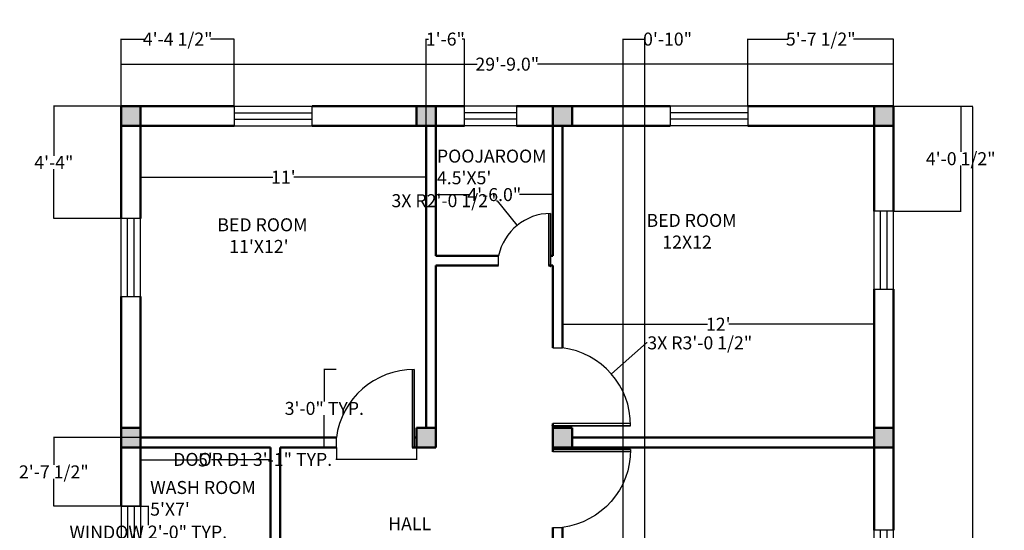
# Model space of a CAD drawing. Units: inches. Extents: x 1935 to 2390, y 6777 to 7449.
# Tile 2 of 2: x 1935 to 2390, y 7213 to 7449. Entities that reach past the tile are written whole.
import ezdxf

# ---------------------------------------------------------------- set-up
doc = ezdxf.new("R2010")
doc.units = ezdxf.units.IN
doc.header["$MEASUREMENT"] = 0
for name, color, linetype, lineweight in [('A-ANNO-DIMS', 7, 'Continuous', 18), ('A-AREA-IDEN', 7, 'Continuous', 25), ('A-COLS', 42, 'Continuous', 50), ('A-COLS-PATT', 7, 'Continuous', 13), ('A-DOOR', 50, 'Continuous', 25), ('A-GLAZ', 140, 'Continuous', 25), ('A-WALL', 42, 'Continuous', 50)]:
    doc.layers.add(name, color=color, linetype=linetype, lineweight=lineweight)
doc.styles.get("Standard").update_dxf_attribs({"font": 'arial.ttf'})
doc.dimstyles.get("Standard").update_dxf_attribs({"dimtxt": 6, "dimasz": 0.18, "dimexe": 0.18, "dimexo": 0.0625, "dimgap": 0.09, "dimtad": 0, "dimtih": 1, "dimtoh": 1, "dimdec": 1, "dimzin": 0, "dimdsep": 46, "dimlunit": 3, "dimtxsty": 'Standard', "dimcen": 0.09, "dimclrd": 200, "dimclre": 200, "dimclrt": 200, "dimadec": 0, "dimazin": 0, "dimtfac": 1, "dimtdec": 1, "dimtofl": 0, "dimtmove": 0, "dimatfit": 3, "dimfxl": 1, "dimtolj": 1, "dimtzin": 0, "dimarcsym": 0})

# ---------------------------------------------------------------- blocks, each defined once
blk = doc.blocks.new('*D1')
at = {"layer": 'A-ANNO-DIMS', "color": 0, "lineweight": -2, "transparency": 16777216}
for p, q in [((1990.87, 7400.15), (1990.87, 7376.35)), ((2122.87, 7400.15), (2122.87, 7376.35)), ((1991.05, 7376.53), (2051.97, 7376.53)), ((2122.69, 7376.53), (2061.76, 7376.53))]:
    blk.add_line(p, q, dxfattribs=at)
at = {"layer": 'A-ANNO-DIMS', "color": 0, "transparency": 16777216}
for points in [[(1991.05, 7376.56), (1991.05, 7376.5), (1990.87, 7376.53)], [(2122.69, 7376.56), (2122.69, 7376.5), (2122.87, 7376.53)]]:
    blk.add_solid(points, dxfattribs=at)
at = {"layer": 'Defpoints', "color": 0, "transparency": 16777216}
for p in [(1990.87, 7400.21), (2122.87, 7400.21), (2122.87, 7376.53)]:
    blk.add_point(p, dxfattribs=at)
at = {"layer": 'A-ANNO-DIMS', "color": 0, "transparency": 16777216, "insert": (2056.87, 7376.53), "char_height": 6, "attachment_point": 5}
blk.add_mtext("\\A1;11'", dxfattribs=at)
blk = doc.blocks.new('*D2')
at = {"layer": 'A-ANNO-DIMS', "color": 0, "lineweight": -2, "transparency": 16777216}
for p, q in [((1990.87, 7251.65), (1990.87, 7245.73)), ((2050.87, 7251.65), (2050.87, 7245.73)), ((1991.05, 7245.91), (2018.02, 7245.91)), ((2050.69, 7245.91), (2023.72, 7245.91))]:
    blk.add_line(p, q, dxfattribs=at)
at = {"layer": 'A-ANNO-DIMS', "color": 0, "transparency": 16777216}
for points in [[(1991.05, 7245.94), (1991.05, 7245.88), (1990.87, 7245.91)], [(2050.69, 7245.94), (2050.69, 7245.88), (2050.87, 7245.91)]]:
    blk.add_solid(points, dxfattribs=at)
at = {"layer": 'Defpoints', "color": 0, "transparency": 16777216}
for p in [(1990.87, 7251.71), (2050.87, 7251.71), (2050.87, 7245.91)]:
    blk.add_point(p, dxfattribs=at)
at = {"layer": 'A-ANNO-DIMS', "color": 0, "transparency": 16777216, "insert": (2020.87, 7245.91), "char_height": 6, "attachment_point": 5}
blk.add_mtext("\\A1;5'", dxfattribs=at)
blk = doc.blocks.new('*D7')
at = {"layer": 'A-ANNO-DIMS', "color": 0, "lineweight": -2, "transparency": 16777216}
for p, q in [((2127.37, 7400.15), (2127.37, 7368.27)), ((2181.37, 7400.15), (2181.37, 7368.27)), ((2127.55, 7368.45), (2142.68, 7368.45)), ((2181.19, 7368.45), (2166.05, 7368.45))]:
    blk.add_line(p, q, dxfattribs=at)
at = {"layer": 'A-ANNO-DIMS', "color": 0, "transparency": 16777216}
for points in [[(2127.55, 7368.48), (2127.55, 7368.42), (2127.37, 7368.45)], [(2181.19, 7368.48), (2181.19, 7368.42), (2181.37, 7368.45)]]:
    blk.add_solid(points, dxfattribs=at)
at = {"layer": 'Defpoints', "color": 0, "transparency": 16777216}
for p in [(2127.37, 7400.21), (2181.37, 7400.21), (2181.37, 7368.45)]:
    blk.add_point(p, dxfattribs=at)
at = {"layer": 'A-ANNO-DIMS', "color": 0, "transparency": 16777216, "insert": (2154.37, 7368.45), "char_height": 6, "attachment_point": 5}
blk.add_mtext('\\A1;4\'-6.0"', dxfattribs=at)
blk = doc.blocks.new('*D8')
at = {"layer": 'A-ANNO-DIMS', "color": 0, "lineweight": -2, "transparency": 16777216}
for p, q in [((2185.87, 7316.65), (2185.87, 7308.4)), ((2329.87, 7316.65), (2329.87, 7308.4)), ((2186.05, 7308.58), (2252.97, 7308.58)), ((2329.69, 7308.58), (2262.76, 7308.58))]:
    blk.add_line(p, q, dxfattribs=at)
at = {"layer": 'A-ANNO-DIMS', "color": 0, "transparency": 16777216}
for points in [[(2186.05, 7308.61), (2186.05, 7308.55), (2185.87, 7308.58)], [(2329.69, 7308.61), (2329.69, 7308.55), (2329.87, 7308.58)]]:
    blk.add_solid(points, dxfattribs=at)
at = {"layer": 'Defpoints', "color": 0, "transparency": 16777216}
for p in [(2185.87, 7316.71), (2329.87, 7316.71), (2329.87, 7308.58)]:
    blk.add_point(p, dxfattribs=at)
at = {"layer": 'A-ANNO-DIMS', "color": 0, "transparency": 16777216, "insert": (2257.87, 7308.58), "char_height": 6, "attachment_point": 5}
blk.add_mtext("\\A1;12'", dxfattribs=at)
blk = doc.blocks.new('*D9')
at = {"layer": 'A-ANNO-DIMS', "color": 0, "lineweight": -2, "transparency": 16777216}
for p, q in [((2338.93, 7409.21), (2375.52, 7409.21)), ((2375.34, 7409.03), (2375.34, 7162.62)), ((2375.34, 6909.89), (2375.34, 7156.31)), ((2338.93, 6909.71), (2375.52, 6909.71))]:
    blk.add_line(p, q, dxfattribs=at)
at = {"layer": 'A-ANNO-DIMS', "color": 0, "transparency": 16777216}
for points in [[(2375.31, 7409.03), (2375.37, 7409.03), (2375.34, 7409.21)], [(2375.31, 6909.89), (2375.37, 6909.89), (2375.34, 6909.71)]]:
    blk.add_solid(points, dxfattribs=at)
at = {"layer": 'Defpoints', "color": 0, "transparency": 16777216}
for p in [(2338.87, 7409.21), (2338.87, 6909.71), (2375.34, 6909.71)]:
    blk.add_point(p, dxfattribs=at)
at = {"layer": 'A-ANNO-DIMS', "color": 0, "transparency": 16777216, "insert": (2375.34, 7159.46), "char_height": 6, "attachment_point": 5}
blk.add_mtext('\\A1;41\'-7.5"', dxfattribs=at)
blk = doc.blocks.new('*D10')
at = {"layer": 'A-ANNO-DIMS', "color": 0, "lineweight": -2, "transparency": 16777216}
for p, q in [((1981.87, 7409.28), (1981.87, 7428.86)), ((1982.05, 7428.68), (2146.42, 7428.68)), ((2338.69, 7428.68), (2174.31, 7428.68)), ((2338.87, 7409.28), (2338.87, 7428.86))]:
    blk.add_line(p, q, dxfattribs=at)
at = {"layer": 'A-ANNO-DIMS', "color": 0, "transparency": 16777216}
for points in [[(1982.05, 7428.71), (1982.05, 7428.65), (1981.87, 7428.68)], [(2338.69, 7428.71), (2338.69, 7428.65), (2338.87, 7428.68)]]:
    blk.add_solid(points, dxfattribs=at)
at = {"layer": 'Defpoints', "color": 0, "transparency": 16777216}
for p in [(2338.87, 7428.68), (1981.87, 7409.21), (2338.87, 7409.21)]:
    blk.add_point(p, dxfattribs=at)
at = {"layer": 'A-ANNO-DIMS', "color": 0, "transparency": 16777216, "insert": (2160.37, 7428.68), "char_height": 6, "attachment_point": 5}
blk.add_mtext('\\A1;29\'-9.0"', dxfattribs=at)
blk = doc.blocks.new('WIN-36IN')
for p, q in [((0, 9), (0, 0)), ((0, 9), (36, 9)), ((0, 6), (36, 6)), ((36, 0), (36, 9)), ((0, 3), (36, 3)), ((0, 0), (36, 0))]:
    blk.add_line(p, q)
blk = doc.blocks.new('WIN-24IN')
for p, q in [((0, 24), (9, 24)), ((0, 24), (0, 0)), ((3, 24), (3, 0)), ((6, 24), (6, 0)), ((9, 24), (9, 0)), ((9, 0), (0, 0))]:
    blk.add_line(p, q)
blk = doc.blocks.new('DOOR-SINGLE-36IN')
for p, q in [((0, 37), (4.5, 37)), ((0, 1), (0, 2)), ((36, 2), (0, 2)), ((0, 0), (0, 1)), ((0, 1), (36, 1)), ((36, 1), (0, 1))]:
    blk.add_line(p, q)
blk.add_arc((-0.32, 1), 36.32, 0, 82.3719)
blk = doc.blocks.new('DOOR-SINGLE-24IN')
for p, q in [((23, 24), (23, 0)), ((24, 0), (24, 24)), ((24, 24), (24, 0)), ((0, 0), (0, 4.5)), ((24, 0), (23, 0)), ((25, 0), (24, 0))]:
    blk.add_line(p, q)
blk.add_arc((24, -0.52), 24.52, 90, 168.1877)
blk = doc.blocks.new('*D18')
at = {"layer": 'A-ANNO-DIMS', "color": 200, "lineweight": -2, "transparency": 16777216}
for p, q in [((1990.93, 7224.58), (1994.65, 7224.58)), ((1994.47, 7224.4), (1994.47, 7215.77)), ((1994.47, 7200.76), (1994.47, 7209.39)), ((1990.93, 7200.58), (1994.65, 7200.58))]:
    blk.add_line(p, q, dxfattribs=at)
at = {"layer": 'A-ANNO-DIMS', "color": 200, "transparency": 16777216}
for points in [[(1994.44, 7224.4), (1994.5, 7224.4), (1994.47, 7224.58)], [(1994.44, 7200.76), (1994.5, 7200.76), (1994.47, 7200.58)]]:
    blk.add_solid(points, dxfattribs=at)
at = {"layer": 'Defpoints', "color": 0, "transparency": 16777216}
for p in [(1990.87, 7224.58), (1994.47, 7224.58), (1990.87, 7200.58)]:
    blk.add_point(p, dxfattribs=at)
at = {"layer": 'A-ANNO-DIMS', "color": 200, "transparency": 16777216, "insert": (1994.47, 7212.58), "char_height": 6, "attachment_point": 5}
blk.add_mtext('\\A1;WINDOW 2\'-0" TYP.', dxfattribs=at)
blk = doc.blocks.new('*D20')
at = {"layer": 'A-ANNO-DIMS', "color": 200, "lineweight": -2, "transparency": 16777216}
for p, q in [((2081.37, 7251.65), (2081.37, 7245.98)), ((2118.37, 7251.65), (2118.37, 7245.98)), ((2081.37, 7246.16), (2081.19, 7246.16)), ((2118.19, 7246.16), (2081.55, 7246.16))]:
    blk.add_line(p, q, dxfattribs=at)
at = {"layer": 'A-ANNO-DIMS', "color": 200, "transparency": 16777216}
for points in [[(2081.55, 7246.19), (2081.55, 7246.13), (2081.37, 7246.16)], [(2118.19, 7246.19), (2118.19, 7246.13), (2118.37, 7246.16)]]:
    blk.add_solid(points, dxfattribs=at)
at = {"layer": 'Defpoints', "color": 0, "transparency": 16777216}
for p in [(2081.37, 7251.71), (2118.37, 7251.71), (2081.37, 7246.16)]:
    blk.add_point(p, dxfattribs=at)
at = {"layer": 'A-ANNO-DIMS', "color": 200, "transparency": 16777216, "insert": (2042.7, 7246.16), "char_height": 6, "attachment_point": 5}
blk.add_mtext('\\A1;DOOR D1 3\'-1" TYP.', dxfattribs=at)
blk = doc.blocks.new('*D21')
at = {"layer": 'A-ANNO-DIMS', "color": 200, "lineweight": -2, "transparency": 16777216}
for p, q in [((2081.3, 7287.71), (2075.64, 7287.71)), ((2075.82, 7287.53), (2075.82, 7272.87)), ((2075.82, 7251.89), (2075.82, 7266.56)), ((2081.3, 7251.71), (2075.64, 7251.71))]:
    blk.add_line(p, q, dxfattribs=at)
at = {"layer": 'A-ANNO-DIMS', "color": 200, "transparency": 16777216}
for points in [[(2075.79, 7287.53), (2075.85, 7287.53), (2075.82, 7287.71)], [(2075.79, 7251.89), (2075.85, 7251.89), (2075.82, 7251.71)]]:
    blk.add_solid(points, dxfattribs=at)
at = {"layer": 'Defpoints', "color": 0, "transparency": 16777216}
for p in [(2075.82, 7287.71), (2081.37, 7287.71), (2081.37, 7251.71)]:
    blk.add_point(p, dxfattribs=at)
at = {"layer": 'A-ANNO-DIMS', "color": 200, "transparency": 16777216, "insert": (2075.82, 7269.71), "char_height": 6, "attachment_point": 5}
blk.add_mtext('\\A1;3\'-0" TYP.', dxfattribs=at)
blk = doc.blocks.new('*D30')
at = {"layer": 'A-ANNO-DIMS', "color": 200, "lineweight": -2, "transparency": 16777216}
for p, q in [((2213.87, 7127.28), (2213.87, 7440.44)), ((2214.05, 7440.26), (2223.69, 7440.26)), ((2223.87, 7127.28), (2223.87, 7440.44)), ((2223.87, 7440.26), (2224.05, 7440.26))]:
    blk.add_line(p, q, dxfattribs=at)
at = {"layer": 'A-ANNO-DIMS', "color": 200, "transparency": 16777216}
for points in [[(2214.05, 7440.29), (2214.05, 7440.23), (2213.87, 7440.26)], [(2223.69, 7440.29), (2223.69, 7440.23), (2223.87, 7440.26)]]:
    blk.add_solid(points, dxfattribs=at)
at = {"layer": 'Defpoints', "color": 0, "transparency": 16777216}
for p in [(2223.87, 7440.26), (2213.87, 7127.21), (2223.87, 7127.21)]:
    blk.add_point(p, dxfattribs=at)
at = {"layer": 'A-ANNO-DIMS', "color": 200, "transparency": 16777216, "insert": (2234.44, 7440.26), "char_height": 6, "attachment_point": 5}
blk.add_mtext('\\A1;0\'-10"', dxfattribs=at)
blk = doc.blocks.new('*D32')
at = {"layer": 'A-ANNO-DIMS', "color": 200, "lineweight": -2, "transparency": 16777216}
for p, q in [((1981.87, 7409.28), (1981.87, 7440.44)), ((1982.05, 7440.26), (1992.87, 7440.26)), ((2034.05, 7440.26), (2023.22, 7440.26)), ((2034.23, 7409.28), (2034.23, 7440.44))]:
    blk.add_line(p, q, dxfattribs=at)
at = {"layer": 'A-ANNO-DIMS', "color": 200, "transparency": 16777216}
for points in [[(1982.05, 7440.29), (1982.05, 7440.23), (1981.87, 7440.26)], [(2034.05, 7440.29), (2034.05, 7440.23), (2034.23, 7440.26)]]:
    blk.add_solid(points, dxfattribs=at)
at = {"layer": 'Defpoints', "color": 0, "transparency": 16777216}
for p in [(2034.23, 7440.26), (1981.87, 7409.21), (2034.23, 7409.21)]:
    blk.add_point(p, dxfattribs=at)
at = {"layer": 'A-ANNO-DIMS', "color": 200, "transparency": 16777216, "insert": (2008.05, 7440.26), "char_height": 6, "attachment_point": 5}
blk.add_mtext('\\A1;4\'-4 1/2"', dxfattribs=at)
blk = doc.blocks.new('*D33')
at = {"layer": 'A-ANNO-DIMS', "color": 200, "lineweight": -2, "transparency": 16777216}
for p, q in [((2122.87, 7400.28), (2122.87, 7440.44)), ((2123.05, 7440.26), (2123.98, 7440.26)), ((2140.48, 7440.26), (2139.54, 7440.26)), ((2140.66, 7400.28), (2140.66, 7440.44))]:
    blk.add_line(p, q, dxfattribs=at)
at = {"layer": 'A-ANNO-DIMS', "color": 200, "transparency": 16777216}
for points in [[(2123.05, 7440.29), (2123.05, 7440.23), (2122.87, 7440.26)], [(2140.48, 7440.29), (2140.48, 7440.23), (2140.66, 7440.26)]]:
    blk.add_solid(points, dxfattribs=at)
at = {"layer": 'Defpoints', "color": 0, "transparency": 16777216}
for p in [(2140.66, 7440.26), (2122.87, 7400.21), (2140.66, 7400.21)]:
    blk.add_point(p, dxfattribs=at)
at = {"layer": 'A-ANNO-DIMS', "color": 200, "transparency": 16777216, "insert": (2131.76, 7440.26), "char_height": 6, "attachment_point": 5}
blk.add_mtext('\\A1;1\'-6"', dxfattribs=at)
blk = doc.blocks.new('*D34')
at = {"layer": 'A-ANNO-DIMS', "color": 200, "lineweight": -2, "transparency": 16777216}
for p, q in [((2271.61, 7409.28), (2271.61, 7440.44)), ((2271.79, 7440.26), (2290.19, 7440.26)), ((2338.69, 7440.26), (2320.3, 7440.26)), ((2338.87, 7409.28), (2338.87, 7440.44))]:
    blk.add_line(p, q, dxfattribs=at)
at = {"layer": 'A-ANNO-DIMS', "color": 200, "transparency": 16777216}
for points in [[(2271.79, 7440.29), (2271.79, 7440.23), (2271.61, 7440.26)], [(2338.69, 7440.29), (2338.69, 7440.23), (2338.87, 7440.26)]]:
    blk.add_solid(points, dxfattribs=at)
at = {"layer": 'Defpoints', "color": 0, "transparency": 16777216}
for p in [(2338.87, 7440.26), (2271.61, 7409.21), (2338.87, 7409.21)]:
    blk.add_point(p, dxfattribs=at)
at = {"layer": 'A-ANNO-DIMS', "color": 200, "transparency": 16777216, "insert": (2305.24, 7440.26), "char_height": 6, "attachment_point": 5}
blk.add_mtext('\\A1;5\'-7 1/2"', dxfattribs=at)
blk = doc.blocks.new('*D35')
at = {"layer": 'A-ANNO-DIMS', "color": 200, "lineweight": -2, "transparency": 16777216}
for p, q in [((2338.93, 7409.21), (2370.1, 7409.21)), ((2369.92, 7409.03), (2369.92, 7388.22)), ((2369.92, 7361.02), (2369.92, 7381.83)), ((2338.93, 7360.84), (2370.1, 7360.84))]:
    blk.add_line(p, q, dxfattribs=at)
at = {"layer": 'A-ANNO-DIMS', "color": 200, "transparency": 16777216}
for points in [[(2369.89, 7409.03), (2369.95, 7409.03), (2369.92, 7409.21)], [(2369.89, 7361.02), (2369.95, 7361.02), (2369.92, 7360.84)]]:
    blk.add_solid(points, dxfattribs=at)
at = {"layer": 'Defpoints', "color": 0, "transparency": 16777216}
for p in [(2338.87, 7409.21), (2369.92, 7409.21), (2338.87, 7360.84)]:
    blk.add_point(p, dxfattribs=at)
at = {"layer": 'A-ANNO-DIMS', "color": 200, "transparency": 16777216, "insert": (2369.92, 7385.03), "char_height": 6, "attachment_point": 5}
blk.add_mtext('\\A1;4\'-0 1/2"', dxfattribs=at)
blk = doc.blocks.new('*D39')
at = {"layer": 'A-ANNO-DIMS', "color": 200, "lineweight": -2, "transparency": 16777216}
for p, q in [((1981.8031, 7409.214628), (1950.6356, 7409.214628)), ((1950.8156, 7409.034628), (1950.8156, 7386.368695)), ((1950.8156, 7357.522762), (1950.8156, 7380.188695)), ((1981.8031, 7357.342762), (1950.6356, 7357.342762))]:
    blk.add_line(p, q, dxfattribs=at)
at = {"layer": 'A-ANNO-DIMS', "color": 200, "transparency": 16777216}
for points in [[(1950.7856, 7409.034628), (1950.8456, 7409.034628), (1950.8156, 7409.214628)], [(1950.7856, 7357.522762), (1950.8456, 7357.522762), (1950.8156, 7357.342762)]]:
    blk.add_solid(points, dxfattribs=at)
at = {"layer": 'Defpoints', "color": 0, "transparency": 16777216}
for p in [(1950.8156, 7409.214628), (1981.8656, 7409.214628), (1981.8656, 7357.342762)]:
    blk.add_point(p, dxfattribs=at)
at = {"layer": 'A-ANNO-DIMS', "color": 200, "transparency": 16777216, "insert": (1950.8156, 7383.278695), "char_height": 6, "attachment_point": 5}
blk.add_mtext('\\A1;4\'-4"', dxfattribs=at)
blk = doc.blocks.new('*D40')
at = {"layer": 'A-ANNO-DIMS', "color": 200, "lineweight": -2, "transparency": 16777216}
for p, q in [((1990.8, 7256.21), (1950.64, 7256.21)), ((1950.82, 7256.03), (1950.82, 7243.59)), ((1950.82, 7224.76), (1950.82, 7237.2)), ((1990.8, 7224.58), (1950.64, 7224.58))]:
    blk.add_line(p, q, dxfattribs=at)
at = {"layer": 'A-ANNO-DIMS', "color": 200, "transparency": 16777216}
for points in [[(1950.79, 7256.03), (1950.85, 7256.03), (1950.82, 7256.21)], [(1950.79, 7224.76), (1950.85, 7224.76), (1950.82, 7224.58)]]:
    blk.add_solid(points, dxfattribs=at)
at = {"layer": 'Defpoints', "color": 0, "transparency": 16777216}
for p in [(1950.82, 7256.21), (1990.87, 7256.21), (1990.87, 7224.58)]:
    blk.add_point(p, dxfattribs=at)
at = {"layer": 'A-ANNO-DIMS', "color": 200, "transparency": 16777216, "insert": (1950.82, 7240.4), "char_height": 6, "attachment_point": 5}
blk.add_mtext('\\A1;2\'-7 1/2"', dxfattribs=at)
blk = doc.blocks.new('*D42')
at = {"layer": 'A-ANNO-DIMS', "color": 200, "lineweight": -2, "transparency": 16777216}
for p, q in [((2224.78, 7299.98), (2208.51, 7285.75)), ((2224.96, 7299.98), (2224.78, 7299.98)), ((2180.95, 7261.71), (2181.13, 7261.71)), ((2181.04, 7261.62), (2181.04, 7261.8))]:
    blk.add_line(p, q, dxfattribs=at)
at = {"layer": 'A-ANNO-DIMS', "color": 200, "transparency": 16777216}
blk.add_solid([(2208.49, 7285.77), (2208.53, 7285.73), (2208.38, 7285.63)], dxfattribs=at)
at = {"layer": 'Defpoints', "color": 0, "transparency": 16777216}
for p in [(2208.38, 7285.63), (2181.04, 7261.71)]:
    blk.add_point(p, dxfattribs=at)
at = {"layer": 'A-ANNO-DIMS', "color": 200, "transparency": 16777216, "insert": (2249.33, 7299.98), "char_height": 6, "attachment_point": 5}
blk.add_mtext('\\A1;3X R3\'-0 1/2"', dxfattribs=at)
blk = doc.blocks.new('*D44')
at = {"layer": 'A-ANNO-DIMS', "color": 200, "lineweight": -2, "transparency": 16777216}
for p, q in [((2155.45, 7365.64), (2155.63, 7365.64)), ((2155.63, 7365.64), (2164.79, 7354.36)), ((2180.28, 7335.2), (2180.46, 7335.2)), ((2180.37, 7335.11), (2180.37, 7335.29))]:
    blk.add_line(p, q, dxfattribs=at)
at = {"layer": 'A-ANNO-DIMS', "color": 200, "transparency": 16777216}
blk.add_solid([(2164.81, 7354.38), (2164.77, 7354.35), (2164.9, 7354.23)], dxfattribs=at)
at = {"layer": 'Defpoints', "color": 0, "transparency": 16777216}
for p in [(2164.9, 7354.23), (2180.37, 7335.2)]:
    blk.add_point(p, dxfattribs=at)
at = {"layer": 'A-ANNO-DIMS', "color": 200, "transparency": 16777216, "insert": (2131.08, 7365.64), "char_height": 6, "attachment_point": 5}
blk.add_mtext('\\A1;3X R2\'-0 1/2"', dxfattribs=at)

msp = doc.modelspace()

# ---------------------------------------------------------------- hatches: boundary and pattern name
at = {"layer": 'A-COLS-PATT'}
h = msp.add_hatch(color=256, dxfattribs=at)
h.dxf.hatch_style = 1
h.paths.add_polyline_path([(1990.87, 7409.21), (1981.87, 7409.21), (1981.87, 7400.21), (1990.87, 7400.21)])
h.paths.add_polyline_path([(2127.37, 7409.21), (2118.37, 7409.21), (2118.37, 7400.21), (2127.37, 7400.21)])
h.paths.add_polyline_path([(2190.37, 7409.21), (2181.37, 7409.21), (2181.37, 7400.21), (2190.37, 7400.21)])
h.paths.add_polyline_path([(2338.87, 7409.21), (2329.87, 7409.21), (2329.87, 7400.21), (2338.87, 7400.21)])
h.paths.add_polyline_path([(1990.87, 7260.71), (1981.87, 7260.71), (1981.87, 7251.71), (1990.87, 7251.71)])
h.paths.add_polyline_path([(2127.37, 7260.71), (2118.37, 7260.71), (2118.37, 7251.71), (2127.37, 7251.71)])
h.paths.add_polyline_path([(2190.37, 7260.71), (2181.37, 7260.71), (2181.37, 7251.71), (2190.37, 7251.71)])
h.paths.add_polyline_path([(2338.87, 7260.71), (2329.87, 7260.71), (2329.87, 7251.71), (2338.87, 7251.71)])
h.paths.add_polyline_path([(1990.87, 7131.71), (1981.87, 7131.71), (1981.87, 7122.71), (1990.87, 7122.71)])
h.paths.add_polyline_path([(2127.37, 7131.71), (2118.37, 7131.71), (2118.37, 7122.71), (2127.37, 7122.71)])
h.paths.add_polyline_path([(1990.87, 7047.71), (1981.87, 7047.71), (1981.87, 7038.71), (1990.87, 7038.71)])
h.paths.add_polyline_path([(2127.37, 7047.71), (2118.37, 7047.71), (2118.37, 7038.71), (2127.37, 7038.71)])
h.paths.add_polyline_path([(1990.87, 6918.71), (1981.87, 6918.71), (1981.87, 6909.71), (1990.87, 6909.71)])
h.paths.add_polyline_path([(2131.87, 6918.71), (2122.87, 6918.71), (2122.87, 6909.71), (2131.87, 6909.71)])
h.paths.add_polyline_path([(2190.37, 6918.71), (2181.37, 6918.71), (2181.37, 6909.71), (2190.37, 6909.71)])
h.paths.add_polyline_path([(2338.87, 6918.71), (2329.87, 6918.71), (2329.87, 6909.71), (2338.87, 6909.71)])
h.paths.add_polyline_path([(2190.37, 7047.71), (2181.37, 7047.71), (2181.37, 7038.71), (2190.37, 7038.71)])
h.paths.add_polyline_path([(2338.87, 7047.71), (2329.87, 7047.71), (2329.87, 7038.71), (2338.87, 7038.71)])
h.paths.add_polyline_path([(2190.37, 7131.71), (2181.37, 7131.71), (2181.37, 7122.71), (2190.37, 7122.71)])
h.paths.add_polyline_path([(2338.87, 7131.71), (2329.87, 7131.71), (2329.87, 7122.71), (2338.87, 7122.71)])

# ---------------------------------------------------------------- linework, layer by layer
at = {"layer": 'A-COLS'}
for p, q in [((2127.37, 7409.21), (2118.37, 7409.21)), ((2118.37, 7409.21), (2118.37, 7400.21)), ((2181.37, 7409.21), (2190.37, 7409.21)), ((2190.37, 7409.21), (2190.37, 7400.21)), ((1981.87, 7251.71), (1981.87, 7260.71)), ((1981.87, 7260.71), (1990.87, 7260.71)), ((2127.37, 7260.71), (2118.37, 7260.71)), ((2118.37, 7260.71), (2118.37, 7251.71)), ((2127.37, 7251.71), (2127.37, 7260.71)), ((2181.37, 7251.71), (2181.37, 7260.71)), ((2181.37, 7260.71), (2190.37, 7260.71)), ((2190.37, 7260.71), (2190.37, 7251.71)), ((2329.87, 7251.71), (2329.87, 7260.71)), ((2329.87, 7260.71), (2338.87, 7260.71))]:
    msp.add_line(p, q, dxfattribs=at)
at = {"layer": 'A-DOOR'}
msp.add_line((2118.37, 7251.71), (2116.37, 7251.71), dxfattribs=at)
at = {"layer": 'A-GLAZ'}
msp.add_line((2329.87, 7324.84), (2329.87, 7324.84), dxfattribs=at)
at = {"layer": 'A-WALL'}
for p, q in [((1981.87, 7409.21), (2034.23, 7409.21)), ((1981.87, 7409.21), (1981.87, 7357.34)), ((1990.87, 7409.21), (1990.87, 7357.34)), ((2070.23, 7409.21), (2140.66, 7409.21)), ((2127.37, 7409.21), (2127.37, 7340.21)), ((2164.66, 7409.21), (2235.61, 7409.21)), ((2181.37, 7409.21), (2181.37, 7340.21)), ((2271.61, 7409.21), (2338.87, 7409.21)), ((2329.87, 7409.21), (2329.87, 7360.84)), ((2338.87, 7409.21), (2338.87, 7360.84)), ((1981.87, 7400.21), (2034.23, 7400.21)), ((2070.23, 7400.21), (2140.66, 7400.21)), ((2122.87, 7400.21), (2122.87, 7260.71)), ((2164.66, 7400.21), (2235.61, 7400.21)), ((2185.87, 7400.21), (2185.87, 7297.71)), ((2271.61, 7400.21), (2338.87, 7400.21)), ((2127.37, 7340.21), (2156.37, 7340.21)), ((2180.37, 7340.21), (2181.37, 7340.21)), ((2127.37, 7335.71), (2156.37, 7335.71)), ((2127.37, 7335.71), (2127.37, 7251.71)), ((2179.37, 7335.71), (2181.37, 7335.71)), ((2181.37, 7335.71), (2181.37, 7297.71)), ((2329.87, 7324.84), (2329.87, 7213.42)), ((2338.87, 7324.84), (2338.87, 7213.42)), ((1981.87, 7321.34), (1981.87, 7224.58)), ((1990.87, 7321.34), (1990.87, 7224.58)), ((2181.37, 7262.71), (2181.37, 7249.71)), ((2185.87, 7261.71), (2185.87, 7260.71)), ((1990.87, 7256.21), (2081.37, 7256.21)), ((2117.37, 7256.21), (2118.37, 7256.21)), ((2190.37, 7256.21), (2329.87, 7256.21)), ((1981.87, 7251.71), (2050.87, 7251.71)), ((2050.87, 7251.71), (2050.87, 7167.71)), ((2055.37, 7251.71), (2055.37, 7163.21)), ((2055.37, 7251.71), (2081.37, 7251.71)), ((2116.37, 7251.71), (2127.37, 7251.71)), ((2181.37, 7251.71), (2338.87, 7251.71)), ((2181.37, 7214.71), (2181.37, 7127.21)), ((2185.87, 7214.71), (2185.87, 7131.71))]:
    msp.add_line(p, q, dxfattribs=at)

# ---------------------------------------------------------------- block references
at = {"layer": 'A-DOOR'}
for name, p in [('DOOR-SINGLE-24IN', (2156.37, 7335.72)), ('DOOR-SINGLE-36IN', (2181.37, 7260.72))]:
    msp.add_blockref(name, p, dxfattribs=at)
at = {"layer": 'A-DOOR', "rotation": 89.9999999999987}
msp.add_blockref('DOOR-SINGLE-36IN', (2118.37, 7251.72), dxfattribs=at)
at = {"layer": 'A-DOOR', "extrusion": (0, 0, -1), "zscale": -1, "rotation": 180}
msp.add_blockref('DOOR-SINGLE-36IN', (-2181.37, 7251.71), dxfattribs=at)
at = {"layer": 'A-GLAZ'}
for name, p in [('WIN-36IN', (2034.23, 7400.22)), ('WIN-24IN', (1981.87, 7200.58))]:
    msp.add_blockref(name, p, dxfattribs=at)
for name, p, rotation in [('WIN-24IN', (2140.66, 7409.21), 270.0000000000007), ('WIN-36IN', (2271.62, 7409.21), 180), ('WIN-36IN', (2338.87, 7324.84), 90.00000000000374), ('WIN-36IN', (1990.87, 7321.34), 90.00000000000374), ('WIN-36IN', (2338.87, 7177.42), 90.00000000000443)]:
    msp.add_blockref(name, p, dxfattribs=dict(at, rotation=rotation))

# ---------------------------------------------------------------- texts
at = {"layer": 'A-AREA-IDEN', "char_height": 6, "attachment_point": 1}
for s, width, insert in [("POOJAROOM\\P4.5'X5'", 51.6974, (2127.86, 7389.22)), ('BED ROOM\\P    12X12', 80.8487, (2224.7, 7359.53)), ("BED ROOM\\P   11'X12'", 72.7958, (2026.39, 7357.5)), ("WASH ROOM\\P5'X7'", 116.3781, (1995.33, 7236.18)), ("HALL\\P10.5'X10'", 47.0238, (2105.34, 7219.45))]:
    msp.add_mtext_dynamic_manual_height_columns(s, width=width, gutter_width=30, heights=[0], dxfattribs=dict(at, insert=insert))

# ---------------------------------------------------------------- dimensions: what is measured, and where the dimension line sits
at = {"layer": 'A-ANNO-DIMS'}
for base, p1, p2, override, picture, middle in [((2034.23, 7440.26), (1981.87, 7409.21), (2034.23, 7409.21), {"dimdec": 1, "dimlfac": 1, "dimrnd": 0, "dimzin": 1, "dimdsep": 46, "dimlunit": 4, "dimfrac": 2}, '*D32', (2008.05, 7440.26)), ((2338.87, 7440.26), (2271.61, 7409.21), (2338.87, 7409.21), {"dimdec": 1, "dimlfac": 1, "dimrnd": 0, "dimzin": 1, "dimdsep": 46, "dimlunit": 4, "dimfrac": 2}, '*D34', (2305.24, 7440.26)), ((2140.66, 7440.26), (2122.87, 7400.21), (2140.66, 7400.21), {"dimdec": 1, "dimlfac": 1, "dimrnd": 0, "dimzin": 1, "dimdsep": 46, "dimlunit": 4, "dimfrac": 2}, '*D33', (2131.76, 7440.26)), ((2223.87, 7440.26), (2213.87, 7127.21), (2223.87, 7127.21), {"dimdec": 1, "dimlfac": 1, "dimrnd": 0, "dimzin": 1, "dimdsep": 46, "dimlunit": 4, "dimfrac": 2}, '*D30', (2234.44, 7440.26)), ((2338.87, 7428.68), (1981.87, 7409.21), (2338.87, 7409.21), {"dimclrd": 0, "dimclre": 0, "dimclrt": 0}, '*D10', (2160.37, 7428.68)), ((2122.87, 7376.53), (1990.87, 7400.21), (2122.87, 7400.21), {"dimclrd": 0, "dimclre": 0, "dimclrt": 0}, '*D1', (2056.87, 7376.53)), ((2181.37, 7368.45), (2127.37, 7400.21), (2181.37, 7400.21), {"dimclrd": 0, "dimclre": 0, "dimclrt": 0}, '*D7', (2154.37, 7368.45)), ((2329.87, 7308.58), (2185.87, 7316.71), (2329.87, 7316.71), {"dimclrd": 0, "dimclre": 0, "dimclrt": 0}, '*D8', (2257.87, 7308.58)), ((2050.87, 7245.91), (1990.87, 7251.71), (2050.87, 7251.71), {"dimclrd": 0, "dimclre": 0, "dimclrt": 0}, '*D2', (2020.87, 7245.91))]:
    dim = msp.add_linear_dim(base=base, p1=p1, p2=p2, dimstyle='Standard', override=override, dxfattribs=at)
    dim.commit()
    dim.dimension.update_dxf_attribs({"geometry": picture, "text_midpoint": middle})
for base, p1, p2, override, picture, middle in [((1950.82, 7409.21), (1981.87, 7357.34), (1981.87, 7409.21), {"dimdec": 1, "dimlfac": 1, "dimrnd": 0, "dimzin": 1, "dimdsep": 46, "dimlunit": 4, "dimfrac": 2}, '*D39', (1950.82, 7383.28)), ((2375.34, 6909.71), (2338.87, 7409.21), (2338.87, 6909.71), {"dimclrd": 0, "dimclre": 0, "dimclrt": 0}, '*D9', (2375.34, 7159.46)), ((2369.92, 7409.21), (2338.87, 7360.84), (2338.87, 7409.21), {"dimdec": 1, "dimlfac": 1, "dimrnd": 0, "dimzin": 1, "dimdsep": 46, "dimlunit": 4, "dimfrac": 2}, '*D35', (2369.92, 7385.03)), ((1950.82, 7256.21), (1990.87, 7224.58), (1990.87, 7256.21), {"dimdec": 1, "dimlfac": 1, "dimrnd": 0, "dimzin": 1, "dimdsep": 46, "dimlunit": 4, "dimfrac": 2}, '*D40', (1950.82, 7240.4))]:
    dim = msp.add_linear_dim(base=base, p1=p1, p2=p2, angle=90, dimstyle='Standard', override=override, dxfattribs=at)
    dim.commit()
    dim.dimension.update_dxf_attribs({"geometry": picture, "text_midpoint": middle})
for center, mpoint, picture, middle in [((2180.37, 7335.2), (2164.9, 7354.23), '*D44', (2131.08, 7365.64)), ((2181.04, 7261.71), (2208.38, 7285.63), '*D42', (2249.33, 7299.98))]:
    dim = msp.add_radius_dim(center=center, mpoint=mpoint, text='3X <>', dimstyle='Standard', override={"dimdec": 1, "dimlfac": 1, "dimrnd": 0, "dimzin": 1, "dimdsep": 46, "dimlunit": 4, "dimfrac": 2}, dxfattribs=at)
    dim.commit()
    dim.dimension.update_dxf_attribs({"geometry": picture, "text_midpoint": middle, "dimtype": 164})
for base, p1, p2, angle, text, picture, middle in [((2075.82, 7287.71), (2081.37, 7251.71), (2081.37, 7287.71), 90, '<> TYP.', '*D21', (2075.82, 7269.71)), ((2081.37, 7246.16), (2118.37, 7251.71), (2081.37, 7251.71), 180, 'DOOR D1 <> TYP.', '*D20', (2042.7, 7246.16)), ((1994.47, 7224.58), (1990.87, 7200.58), (1990.87, 7224.58), 90, 'WINDOW <> TYP.', '*D18', (1994.47, 7212.58))]:
    dim = msp.add_linear_dim(base=base, p1=p1, p2=p2, angle=angle, text=text, dimstyle='Standard', override={"dimdec": 1, "dimlfac": 1, "dimrnd": 0, "dimzin": 1, "dimdsep": 46, "dimlunit": 4, "dimfrac": 2}, dxfattribs=at)
    dim.commit()
    dim.dimension.update_dxf_attribs({"geometry": picture, "text_midpoint": middle})

doc.saveas('drawing.dxf')
